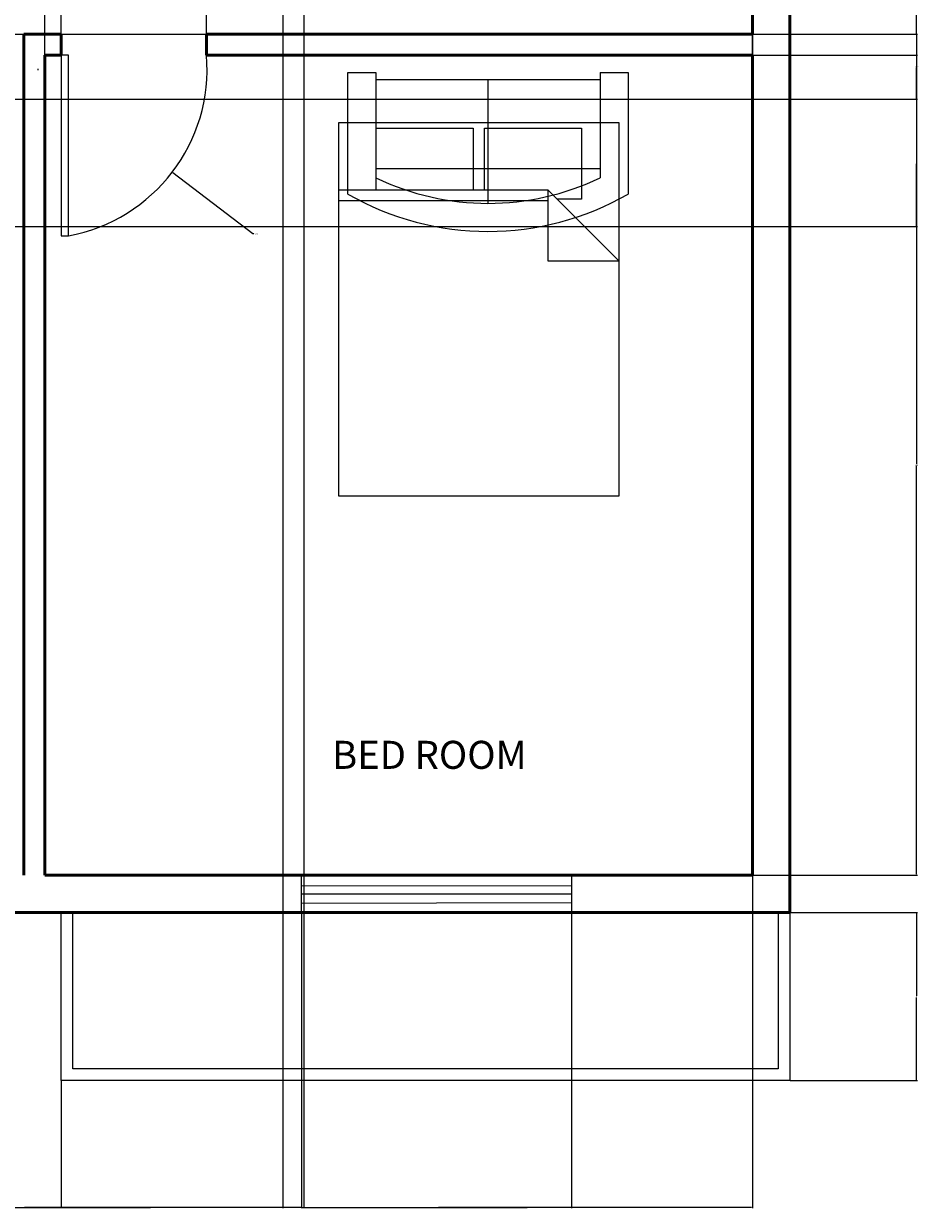
# Model space of a CAD drawing. Units: inches. Extents: x 2907 to 3328, y 1715 to 2286.
# Tile 2 of 5: x 3137 to 3328, y 1715 to 1969. Entities that reach past the tile are written whole.
import ezdxf

# ---------------------------------------------------------------- set-up
doc = ezdxf.new("R2010")
doc.units = ezdxf.units.IN
for name, color, linetype, lineweight in [('A-ANNO-DIMS', 2, 'Continuous', 18), ('A-AREA-IDEN', 7, 'Continuous', 25), ('A-DOOR', 3, 'Continuous', 25), ('A-FLOR-OTLN', 7, 'Continuous', 25), ('A-FURN', 8, 'Continuous', 18), ('A-GLAZ', 4, 'Continuous', 18), ('A-WALL', 7, 'Continuous', 50)]:
    doc.layers.add(name, color=color, linetype=linetype, lineweight=lineweight)
doc.styles.get("Standard").update_dxf_attribs({"font": 'arial.ttf'})
doc.dimstyles.get("Standard").update_dxf_attribs({"dimtxt": 0.18, "dimasz": 0.18, "dimexe": 0.18, "dimexo": 0.0625, "dimgap": 0.09, "dimtad": 0, "dimtih": 1, "dimtoh": 1, "dimdec": 4, "dimzin": 0, "dimdsep": 46, "dimtxsty": 'Standard', "dimcen": 0.09, "dimadec": 0, "dimazin": 0, "dimtfac": 1, "dimtdec": 4, "dimtofl": 0, "dimtmove": 0, "dimatfit": 3, "dimfxl": 1, "dimtolj": 1, "dimtzin": 0, "dimarcsym": 0})

# ---------------------------------------------------------------- blocks, each defined once
blk = doc.blocks.new('Bed - Queen')
for p, q in [((0, -80.00003), (0, 0)), ((0, 0), (59.99999, 0)), ((59.99999, 0), (59.99999, -80.00003)), ((7.99999, -1.2), (28.79998, -1.2)), ((7.99999, -14.4), (7.99999, -1.2)), ((28.79998, -1.2), (28.79998, -14.4)), ((31.19999, -1.2), (51.99999, -1.2)), ((31.19999, -14.4), (31.19999, -1.2)), ((51.99999, -1.2), (51.99999, -16.4)), ((0, -14.4), (44.8, -14.4)), ((59.99999, -29.6), (44.8, -14.4)), ((44.8, -14.4), (44.8, -29.6)), ((44.8, -16.8), (0, -16.8)), ((51.99999, -16.4), (46.79936, -16.4)), ((44.8, -29.6), (59.99999, -29.6)), ((59.99999, -80.00003), (0, -80.00003))]:
    blk.add_line(p, q)
blk = doc.blocks.new('Sofa - Roundback Loveseat 5 ft.')
for p, q in [((0, -32.44198), (0, -5.99998)), ((-24, -33.99998), (-24, -11.46958)), ((24.00004, -33.99998), (24.00004, -11.46958)), ((-23.9998, -13.38178), (23.99986, -13.38178)), ((-24, -32.44198), (24.00004, -32.44198))]:
    blk.add_line(p, q)
for points in [[(-24, -33.99998), (-30, -33.99998), (-30, -7.99998)], [(30.00004, -7.99998), (30.00004, -33.99998), (24.00004, -33.99998)]]:
    blk.add_lwpolyline(points)
for centre, radius, start, end in [((0, -60.24998), 60.24998, 60.13715, 119.8628), ((0, -61.38438), 55.38444, 64.32083, 115.6792)]:
    blk.add_arc(centre, radius, start, end)
blk = doc.blocks.new('*D15')
at = {"layer": 'A-ANNO-DIMS', "color": 0, "lineweight": -2, "transparency": 16777216}
for p, q in [((3300.65, 1778.83), (3327.92, 1778.83)), ((3327.74, 1778.65), (3327.74, 1761.01)), ((3327.74, 1743.01), (3327.74, 1760.65)), ((3300.65, 1742.83), (3327.92, 1742.83))]:
    blk.add_line(p, q, dxfattribs=at)
at = {"layer": 'A-ANNO-DIMS', "color": 0, "transparency": 16777216}
for points in [[(3327.71, 1778.65), (3327.77, 1778.65), (3327.74, 1778.83)], [(3327.71, 1743.01), (3327.77, 1743.01), (3327.74, 1742.83)]]:
    blk.add_solid(points, dxfattribs=at)
at = {"layer": 'Defpoints', "color": 0, "transparency": 16777216}
for p in [(3300.59, 1778.83), (3327.74, 1778.83), (3300.59, 1742.83)]:
    blk.add_point(p, dxfattribs=at)
at = {"layer": 'A-ANNO-DIMS', "color": 0, "transparency": 16777216, "insert": (3327.74, 1760.83), "char_height": 0.18, "attachment_point": 5}
blk.add_mtext('\\A1;36', dxfattribs=at)
blk = doc.blocks.new('*D17')
at = {"layer": 'A-ANNO-DIMS', "color": 0, "lineweight": -2, "transparency": 16777216}
for p, q in [((3080.59, 2250.77), (3080.59, 1715.5)), ((3192.09, 2250.77), (3192.09, 1715.5)), ((3080.77, 1715.68), (3135.95, 1715.68)), ((3191.91, 1715.68), (3136.73, 1715.68))]:
    blk.add_line(p, q, dxfattribs=at)
at = {"layer": 'A-ANNO-DIMS', "color": 0, "transparency": 16777216}
for points in [[(3080.77, 1715.71), (3080.77, 1715.65), (3080.59, 1715.68)], [(3191.91, 1715.71), (3191.91, 1715.65), (3192.09, 1715.68)]]:
    blk.add_solid(points, dxfattribs=at)
at = {"layer": 'Defpoints', "color": 0, "transparency": 16777216}
for p in [(3080.59, 2250.83), (3192.09, 2250.83), (3192.09, 1715.68)]:
    blk.add_point(p, dxfattribs=at)
at = {"layer": 'A-ANNO-DIMS', "color": 0, "transparency": 16777216, "insert": (3136.34, 1715.68), "char_height": 0.18, "attachment_point": 5}
blk.add_mtext('\\A1;111.5', dxfattribs=at)
blk = doc.blocks.new('*D18')
at = {"layer": 'A-ANNO-DIMS', "color": 0, "lineweight": -2, "transparency": 16777216}
for p, q in [((3196.59, 2250.77), (3196.59, 1715.5)), ((3292.59, 2250.77), (3292.59, 1715.5)), ((3196.77, 1715.68), (3244.37, 1715.68)), ((3292.41, 1715.68), (3244.81, 1715.68))]:
    blk.add_line(p, q, dxfattribs=at)
at = {"layer": 'A-ANNO-DIMS', "color": 0, "transparency": 16777216}
for points in [[(3196.77, 1715.71), (3196.77, 1715.65), (3196.59, 1715.68)], [(3292.41, 1715.71), (3292.41, 1715.65), (3292.59, 1715.68)]]:
    blk.add_solid(points, dxfattribs=at)
at = {"layer": 'Defpoints', "color": 0, "transparency": 16777216}
for p in [(3196.59, 2250.83), (3292.59, 2250.83), (3292.59, 1715.68)]:
    blk.add_point(p, dxfattribs=at)
at = {"layer": 'A-ANNO-DIMS', "color": 0, "transparency": 16777216, "insert": (3244.59, 1715.68), "char_height": 0.18, "attachment_point": 5}
blk.add_mtext('\\A1;96', dxfattribs=at)
blk = doc.blocks.new('*D29')
at = {"layer": 'A-ANNO-DIMS', "color": 0, "lineweight": -2, "transparency": 16777216}
for p, q in [((3292.65, 2102.33), (3327.92, 2102.33)), ((3327.74, 2102.15), (3327.74, 2034.76)), ((3327.74, 1967.01), (3327.74, 2034.4)), ((3292.65, 1966.83), (3327.92, 1966.83))]:
    blk.add_line(p, q, dxfattribs=at)
at = {"layer": 'A-ANNO-DIMS', "color": 0, "transparency": 16777216}
for points in [[(3327.71, 2102.15), (3327.77, 2102.15), (3327.74, 2102.33)], [(3327.71, 1967.01), (3327.77, 1967.01), (3327.74, 1966.83)]]:
    blk.add_solid(points, dxfattribs=at)
at = {"layer": 'Defpoints', "color": 0, "transparency": 16777216}
for p in [(3292.59, 2102.33), (3327.74, 2102.33), (3292.59, 1966.83)]:
    blk.add_point(p, dxfattribs=at)
at = {"layer": 'A-ANNO-DIMS', "color": 0, "transparency": 16777216, "insert": (3327.74, 2034.58), "char_height": 0.18, "attachment_point": 5}
blk.add_mtext('\\A1;135.5', dxfattribs=at)
blk = doc.blocks.new('*D30')
at = {"layer": 'A-ANNO-DIMS', "color": 0, "lineweight": -2, "transparency": 16777216}
for p, q in [((3292.65, 1962.33), (3327.92, 1962.33)), ((3327.74, 1962.15), (3327.74, 1874.76)), ((3327.74, 1787.01), (3327.74, 1874.4)), ((3292.65, 1786.83), (3327.92, 1786.83))]:
    blk.add_line(p, q, dxfattribs=at)
at = {"layer": 'A-ANNO-DIMS', "color": 0, "transparency": 16777216}
for points in [[(3327.71, 1962.15), (3327.77, 1962.15), (3327.74, 1962.33)], [(3327.71, 1787.01), (3327.77, 1787.01), (3327.74, 1786.83)]]:
    blk.add_solid(points, dxfattribs=at)
at = {"layer": 'Defpoints', "color": 0, "transparency": 16777216}
for p in [(3292.59, 1962.33), (3327.74, 1962.33), (3292.59, 1786.83)]:
    blk.add_point(p, dxfattribs=at)
at = {"layer": 'A-ANNO-DIMS', "color": 0, "transparency": 16777216, "insert": (3327.74, 1874.58), "char_height": 0.18, "attachment_point": 5}
blk.add_mtext('\\A1;175.5', dxfattribs=at)
blk = doc.blocks.new('*D32')
at = {"layer": 'A-ANNO-DIMS', "color": 0, "lineweight": -2, "transparency": 16777216}
for p, q in [((3141.09, 1786.89), (3141.09, 2286.16)), ((3141.27, 2285.98), (3216.45, 2285.98)), ((3292.41, 2285.98), (3217.23, 2285.98)), ((3292.59, 1786.89), (3292.59, 2286.16))]:
    blk.add_line(p, q, dxfattribs=at)
at = {"layer": 'A-ANNO-DIMS', "color": 0, "transparency": 16777216}
for points in [[(3141.27, 2286.01), (3141.27, 2285.95), (3141.09, 2285.98)], [(3292.41, 2286.01), (3292.41, 2285.95), (3292.59, 2285.98)]]:
    blk.add_solid(points, dxfattribs=at)
at = {"layer": 'Defpoints', "color": 0, "transparency": 16777216}
for p in [(3292.59, 2285.98), (3141.09, 1786.83), (3292.59, 1786.83)]:
    blk.add_point(p, dxfattribs=at)
at = {"layer": 'A-ANNO-DIMS', "color": 0, "transparency": 16777216, "insert": (3216.84, 2285.98), "char_height": 0.18, "attachment_point": 5}
blk.add_mtext('\\A1;151.5', dxfattribs=at)
blk = doc.blocks.new('*D35')
at = {"layer": 'A-ANNO-DIMS', "color": 0, "lineweight": -2, "transparency": 16777216}
for p, q in [((3131.97, 1778.77), (3131.97, 1715.5)), ((3196.08, 1778.77), (3196.08, 1715.5)), ((3132.15, 1715.68), (3163.72, 1715.68)), ((3195.9, 1715.68), (3164.33, 1715.68))]:
    blk.add_line(p, q, dxfattribs=at)
at = {"layer": 'A-ANNO-DIMS', "color": 0, "transparency": 16777216}
for points in [[(3132.15, 1715.71), (3132.15, 1715.65), (3131.97, 1715.68)], [(3195.9, 1715.71), (3195.9, 1715.65), (3196.08, 1715.68)]]:
    blk.add_solid(points, dxfattribs=at)
at = {"layer": 'Defpoints', "color": 0, "transparency": 16777216}
for p in [(3131.97, 1778.83), (3196.08, 1778.83), (3196.08, 1715.68)]:
    blk.add_point(p, dxfattribs=at)
at = {"layer": 'A-ANNO-DIMS', "color": 0, "transparency": 16777216, "insert": (3164.03, 1715.68), "char_height": 0.18, "attachment_point": 5}
blk.add_mtext('\\A1;64.1', dxfattribs=at)
blk = doc.blocks.new('*D36')
at = {"layer": 'A-ANNO-DIMS', "color": 0, "lineweight": -2, "transparency": 16777216}
for p, q in [((3196.08, 1778.77), (3196.08, 1715.5)), ((3253.9, 1778.77), (3253.9, 1715.5)), ((3196.26, 1715.68), (3224.6, 1715.68)), ((3253.72, 1715.68), (3225.38, 1715.68))]:
    blk.add_line(p, q, dxfattribs=at)
at = {"layer": 'A-ANNO-DIMS', "color": 0, "transparency": 16777216}
for points in [[(3196.26, 1715.71), (3196.26, 1715.65), (3196.08, 1715.68)], [(3253.72, 1715.71), (3253.72, 1715.65), (3253.9, 1715.68)]]:
    blk.add_solid(points, dxfattribs=at)
at = {"layer": 'Defpoints', "color": 0, "transparency": 16777216}
for p in [(3196.08, 1778.83), (3253.9, 1778.83), (3253.9, 1715.68)]:
    blk.add_point(p, dxfattribs=at)
at = {"layer": 'A-ANNO-DIMS', "color": 0, "transparency": 16777216, "insert": (3224.99, 1715.68), "char_height": 0.18, "attachment_point": 5}
blk.add_mtext('\\A1;57.82', dxfattribs=at)
blk = doc.blocks.new('*D40')
at = {"layer": 'A-ANNO-DIMS', "color": 0, "lineweight": -2, "transparency": 16777216}
for p, q in [((3026.52, 1952.9), (3327.92, 1952.9)), ((3327.74, 1952.72), (3327.74, 1939.45)), ((3327.74, 1925.82), (3327.74, 1939.09)), ((3026.52, 1925.64), (3327.92, 1925.64))]:
    blk.add_line(p, q, dxfattribs=at)
at = {"layer": 'A-ANNO-DIMS', "color": 0, "transparency": 16777216}
for points in [[(3327.71, 1952.72), (3327.77, 1952.72), (3327.74, 1952.9)], [(3327.71, 1925.82), (3327.77, 1925.82), (3327.74, 1925.64)]]:
    blk.add_solid(points, dxfattribs=at)
at = {"layer": 'Defpoints', "color": 0, "transparency": 16777216}
for p in [(3026.46, 1952.9), (3327.74, 1952.9), (3026.46, 1925.64)]:
    blk.add_point(p, dxfattribs=at)
at = {"layer": 'A-ANNO-DIMS', "color": 0, "transparency": 16777216, "insert": (3327.74, 1939.27), "char_height": 0.18, "attachment_point": 5}
blk.add_mtext('\\A1;27.27', dxfattribs=at)
blk = doc.blocks.new('*D41')
at = {"layer": 'A-ANNO-DIMS', "color": 0, "lineweight": -2, "transparency": 16777216}
for p, q in [((3026.52, 1966.83), (3327.92, 1966.83)), ((3327.74, 1966.65), (3327.74, 1960.05)), ((3327.74, 1953.08), (3327.74, 1959.68)), ((3026.52, 1952.9), (3327.92, 1952.9))]:
    blk.add_line(p, q, dxfattribs=at)
at = {"layer": 'A-ANNO-DIMS', "color": 0, "transparency": 16777216}
for points in [[(3327.71, 1966.65), (3327.77, 1966.65), (3327.74, 1966.83)], [(3327.71, 1953.08), (3327.77, 1953.08), (3327.74, 1952.9)]]:
    blk.add_solid(points, dxfattribs=at)
at = {"layer": 'Defpoints', "color": 0, "transparency": 16777216}
for p in [(3026.46, 1966.83), (3327.74, 1966.83), (3026.46, 1952.9)]:
    blk.add_point(p, dxfattribs=at)
at = {"layer": 'A-ANNO-DIMS', "color": 0, "transparency": 16777216, "insert": (3327.74, 1959.87), "char_height": 0.18, "attachment_point": 5}
blk.add_mtext('\\A1;13.927', dxfattribs=at)
blk = doc.blocks.new('*D42')
at = {"layer": 'A-ANNO-DIMS', "color": 0, "lineweight": -2, "transparency": 16777216}
for p, q in [((3144.59, 1966.89), (3144.59, 1994.16)), ((3144.77, 1993.98), (3159.69, 1993.98)), ((3175.54, 1993.98), (3160.62, 1993.98)), ((3175.72, 1966.89), (3175.72, 1994.16))]:
    blk.add_line(p, q, dxfattribs=at)
at = {"layer": 'A-ANNO-DIMS', "color": 0, "transparency": 16777216}
for points in [[(3144.77, 1994.01), (3144.77, 1993.95), (3144.59, 1993.98)], [(3175.54, 1994.01), (3175.54, 1993.95), (3175.72, 1993.98)]]:
    blk.add_solid(points, dxfattribs=at)
at = {"layer": 'Defpoints', "color": 0, "transparency": 16777216}
for p in [(3175.72, 1993.98), (3144.59, 1966.83), (3175.72, 1966.83)]:
    blk.add_point(p, dxfattribs=at)
at = {"layer": 'A-ANNO-DIMS', "color": 0, "transparency": 16777216, "insert": (3160.16, 1993.98), "char_height": 0.18, "attachment_point": 5}
blk.add_mtext('\\A1;31.134', dxfattribs=at)
blk = doc.blocks.new('*D43')
at = {"layer": 'A-ANNO-DIMS', "color": 0, "lineweight": -2, "transparency": 16777216}
for p, q in [((3175.72, 1966.89), (3175.72, 1994.16)), ((3175.9, 1993.98), (3233.7, 1993.98)), ((3292.41, 1993.98), (3234.61, 1993.98)), ((3292.59, 1966.89), (3292.59, 1994.16))]:
    blk.add_line(p, q, dxfattribs=at)
at = {"layer": 'A-ANNO-DIMS', "color": 0, "transparency": 16777216}
for points in [[(3175.9, 1994.01), (3175.9, 1993.95), (3175.72, 1993.98)], [(3292.41, 1994.01), (3292.41, 1993.95), (3292.59, 1993.98)]]:
    blk.add_solid(points, dxfattribs=at)
at = {"layer": 'Defpoints', "color": 0, "transparency": 16777216}
for p in [(3292.59, 1993.98), (3175.72, 1966.83), (3292.59, 1966.83)]:
    blk.add_point(p, dxfattribs=at)
at = {"layer": 'A-ANNO-DIMS', "color": 0, "transparency": 16777216, "insert": (3234.16, 1993.98), "char_height": 0.18, "attachment_point": 5}
blk.add_mtext('\\A1;116.87', dxfattribs=at)
blk = doc.blocks.new('*D49')
at = {"layer": 'A-ANNO-DIMS', "color": 0, "lineweight": -2, "transparency": 16777216}
for p, q in [((3131.97, 1747.6), (3131.97, 1715.5)), ((3144.59, 1742.77), (3144.59, 1715.5)), ((3132.15, 1715.68), (3137.83, 1715.68)), ((3144.41, 1715.68), (3138.74, 1715.68))]:
    blk.add_line(p, q, dxfattribs=at)
at = {"layer": 'A-ANNO-DIMS', "color": 0, "transparency": 16777216}
for points in [[(3132.15, 1715.71), (3132.15, 1715.65), (3131.97, 1715.68)], [(3144.41, 1715.71), (3144.41, 1715.65), (3144.59, 1715.68)]]:
    blk.add_solid(points, dxfattribs=at)
at = {"layer": 'Defpoints', "color": 0, "transparency": 16777216}
for p in [(3131.97, 1747.67), (3144.59, 1742.83), (3144.59, 1715.68)]:
    blk.add_point(p, dxfattribs=at)
at = {"layer": 'A-ANNO-DIMS', "color": 0, "transparency": 16777216, "insert": (3138.28, 1715.68), "char_height": 0.18, "attachment_point": 5}
blk.add_mtext('\\A1;12.616', dxfattribs=at)
blk = doc.blocks.new('*D59')
at = {"layer": 'A-ANNO-DIMS', "color": 0, "lineweight": -2, "transparency": 16777216}
for p, q in [((3139.57, 1959.3), (3139.75, 1959.3)), ((3139.66, 1959.21), (3139.66, 1959.39)), ((3185.65, 1924.1), (3168.54, 1937.19)), ((3185.83, 1924.1), (3185.65, 1924.1))]:
    blk.add_line(p, q, dxfattribs=at)
at = {"layer": 'A-ANNO-DIMS', "color": 0, "transparency": 16777216}
blk.add_solid([(3168.56, 1937.22), (3168.53, 1937.17), (3168.4, 1937.3)], dxfattribs=at)
at = {"layer": 'Defpoints', "color": 0, "transparency": 16777216}
for p in [(3139.66, 1959.3), (3168.4, 1937.3)]:
    blk.add_point(p, dxfattribs=at)
at = {"layer": 'A-ANNO-DIMS', "color": 0, "transparency": 16777216, "insert": (3186.31, 1924.1), "char_height": 0.18, "attachment_point": 5}
blk.add_mtext('\\A1;R36.19', dxfattribs=at)

msp = doc.modelspace()

# ---------------------------------------------------------------- linework, layer by layer
at = {"layer": 'A-DOOR'}
for p, q in [((3144.5892, 1962.3301), (3144.5892, 1923.6923)), ((3146.1554, 1962.3301), (3144.5892, 1962.3301)), ((3146.1554, 1923.6923), (3146.1554, 1962.3301)), ((3144.5892, 1923.6923), (3146.1554, 1923.6923))]:
    msp.add_line(p, q, dxfattribs=at)
msp.add_arc((3139.6605, 1959.2951), 36.1903, 280.33858, 4.810656, dxfattribs=at)
at = {"layer": 'A-FLOR-OTLN'}
for p, q in [((3144.5892, 1742.8301), (3144.5892, 1778.8301)), ((3147.0892, 1745.3301), (3147.0892, 1778.8301)), ((3298.0892, 1778.8301), (3298.0892, 1745.3301)), ((3300.5892, 1778.8301), (3300.5892, 1742.8301)), ((3298.0892, 1745.3301), (3147.0892, 1745.3301)), ((3300.5892, 1742.8301), (3144.5892, 1742.8301))]:
    msp.add_line(p, q, dxfattribs=at)
at = {"layer": 'A-GLAZ'}
for p, q in [((3196.0778, 1784.5768), (3253.9027, 1784.5071)), ((3196.0778, 1782.8301), (3253.9027, 1782.8301)), ((3196.0778, 1780.8146), (3253.9027, 1780.954))]:
    msp.add_line(p, q, dxfattribs=at)
msp.add_lwpolyline([(3196.0778, 1786.8301), (3253.9027, 1786.8301), (3253.9027, 1778.8301), (3196.0778, 1778.8301)], close=True, dxfattribs=at)
at = {"layer": 'A-WALL'}
for p, q in [((3300.5892, 2258.8301), (3300.5892, 1778.8301)), ((3292.5892, 2102.3301), (3292.5892, 1966.8301)), ((3136.5892, 1966.8301), (3136.5892, 1786.8301)), ((3144.5892, 1966.8301), (3136.5892, 1966.8301)), ((3144.5892, 1962.3301), (3144.5892, 1966.8301)), ((3175.7234, 1966.8301), (3292.5892, 1966.8301)), ((3175.7234, 1962.3301), (3175.7234, 1966.8301)), ((3141.0892, 1962.3301), (3141.0892, 1786.8301)), ((3144.5892, 1962.3301), (3141.0892, 1962.3301)), ((3175.7234, 1962.3301), (3292.5892, 1962.3301)), ((3292.5892, 1962.3301), (3292.5892, 1786.8301)), ((3292.5892, 1786.8301), (3141.0892, 1786.8301)), ((3300.5892, 1778.8301), (3131.9734, 1778.8301))]:
    msp.add_line(p, q, dxfattribs=at)

# ---------------------------------------------------------------- block references
at = {"layer": 'A-FURN', "rotation": 180}
msp.add_blockref('Sofa - Roundback Loveseat 5 ft.', (3235.9887, 1924.6172), dxfattribs=at)
at = {"layer": 'A-FURN'}
msp.add_blockref('Bed - Queen', (3204.0224, 1947.9301), dxfattribs=at)

# ---------------------------------------------------------------- texts
at = {"layer": 'A-AREA-IDEN', "insert": (3202.6102, 1815.5691), "char_height": 6, "attachment_point": 1}
msp.add_mtext_dynamic_manual_height_columns('BED ROOM ', width=50.965346, gutter_width=12.5, heights=[0], dxfattribs=at)

# ---------------------------------------------------------------- dimensions: what is measured, and where the dimension line sits
at = {"layer": 'A-ANNO-DIMS'}
for base, p1, p2, override, picture, middle in [((3292.5892, 2285.9816), (3141.0892, 1786.8301), (3292.5892, 1786.8301), {"dimdec": 1, "dimlfac": 1, "dimrnd": 0, "dimzin": 0, "dimdsep": 46, "dimlunit": 2}, '*D32', (3216.8392, 2285.9816)), ((3192.0892, 1715.6786), (3080.5892, 2250.8301), (3192.0892, 2250.8301), {"dimdec": 1, "dimlfac": 1, "dimrnd": 0, "dimzin": 0, "dimdsep": 46, "dimlunit": 2}, '*D17', (3136.3392, 1715.6786)), ((3292.5892, 1715.6786), (3196.5892, 2250.8301), (3292.5892, 2250.8301), {"dimdec": 0, "dimlfac": 1, "dimrnd": 0, "dimzin": 0, "dimdsep": 46, "dimlunit": 2}, '*D18', (3244.5892, 1715.6786)), ((3175.7234, 1993.9816), (3144.5892, 1966.8301), (3175.7234, 1966.8301), {"dimdec": 3, "dimlfac": 1, "dimrnd": 0, "dimzin": 0, "dimdsep": 46, "dimlunit": 2}, '*D42', (3160.1563, 1993.9816)), ((3196.0778, 1715.6786), (3131.9734, 1778.8301), (3196.0778, 1778.8301), {"dimdec": 1, "dimlfac": 1, "dimrnd": 0, "dimzin": 0, "dimdsep": 46, "dimlunit": 2}, '*D35', (3164.0256, 1715.6786)), ((3253.9027, 1715.6786), (3196.0778, 1778.8301), (3253.9027, 1778.8301), {"dimdec": 2, "dimlfac": 1, "dimrnd": 0, "dimzin": 0, "dimdsep": 46, "dimlunit": 2}, '*D36', (3224.9902, 1715.6786)), ((3144.5892, 1715.6786), (3131.9734, 1747.6674), (3144.5892, 1742.8301), {"dimdec": 3, "dimlfac": 1, "dimrnd": 0, "dimzin": 0, "dimdsep": 46, "dimlunit": 2}, '*D49', (3138.2813, 1715.6786))]:
    dim = msp.add_linear_dim(base=base, p1=p1, p2=p2, dimstyle='Standard', override=override, dxfattribs=at)
    dim.commit()
    dim.dimension.update_dxf_attribs({"geometry": picture, "text_midpoint": middle})
for base, p1, p2, angle, override, picture, middle in [((3327.7407, 2102.3301), (3292.5892, 1966.8301), (3292.5892, 2102.3301), 90, {"dimdec": 1, "dimlfac": 1, "dimrnd": 0, "dimzin": 0, "dimdsep": 46, "dimlunit": 2}, '*D29', (3327.7407, 2034.5801)), ((3292.5892, 1993.9816), (3175.7234, 1966.8301), (3292.5892, 1966.8301), 0, {"dimdec": 2, "dimlfac": 1, "dimrnd": 0, "dimzin": 0, "dimdsep": 46, "dimlunit": 2}, '*D43', (3234.1563, 1993.9816)), ((3327.74068, 1966.8301), (3026.46005, 1952.90358), (3026.46005, 1966.8301), 90, {"dimdec": 3, "dimlfac": 1, "dimrnd": 0, "dimzin": 0, "dimdsep": 46, "dimlunit": 2}, '*D41', (3327.74068, 1959.86684)), ((3327.7407, 1962.3301), (3292.5892, 1786.8301), (3292.5892, 1962.3301), 90, {"dimdec": 1, "dimlfac": 1, "dimrnd": 0, "dimzin": 0, "dimdsep": 46, "dimlunit": 2}, '*D30', (3327.7407, 1874.5801)), ((3327.7407, 1952.9036), (3026.46, 1925.6352), (3026.46, 1952.9036), 90, {"dimdec": 2, "dimlfac": 1, "dimrnd": 0, "dimzin": 0, "dimdsep": 46, "dimlunit": 2}, '*D40', (3327.7407, 1939.2694)), ((3327.7407, 1778.8301), (3300.5892, 1742.8301), (3300.5892, 1778.8301), 90, {"dimdec": 0, "dimlfac": 1, "dimrnd": 0, "dimzin": 0, "dimdsep": 46, "dimlunit": 2}, '*D15', (3327.7407, 1760.8301))]:
    dim = msp.add_linear_dim(base=base, p1=p1, p2=p2, angle=angle, dimstyle='Standard', override=override, dxfattribs=at)
    dim.commit()
    dim.dimension.update_dxf_attribs({"geometry": picture, "text_midpoint": middle})
dim = msp.add_radius_dim(center=(3139.6605, 1959.2951), mpoint=(3168.4009, 1937.3011), dimstyle='Standard', override={"dimdec": 2, "dimlfac": 1, "dimrnd": 0, "dimzin": 0, "dimdsep": 46, "dimlunit": 2}, dxfattribs=at)
dim.commit()
dim.dimension.update_dxf_attribs({"geometry": '*D59', "text_midpoint": (3186.3051, 1924.1047), "dimtype": 164})

doc.saveas('drawing.dxf')
